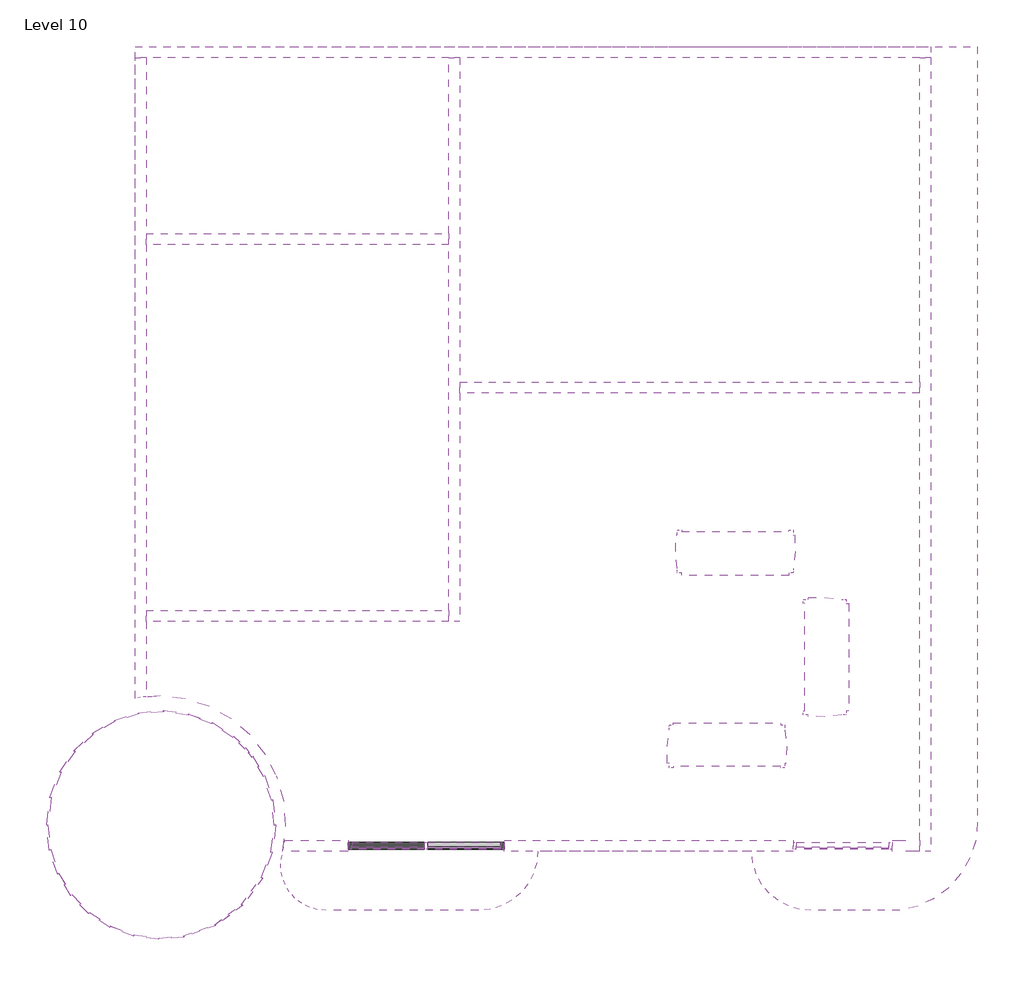
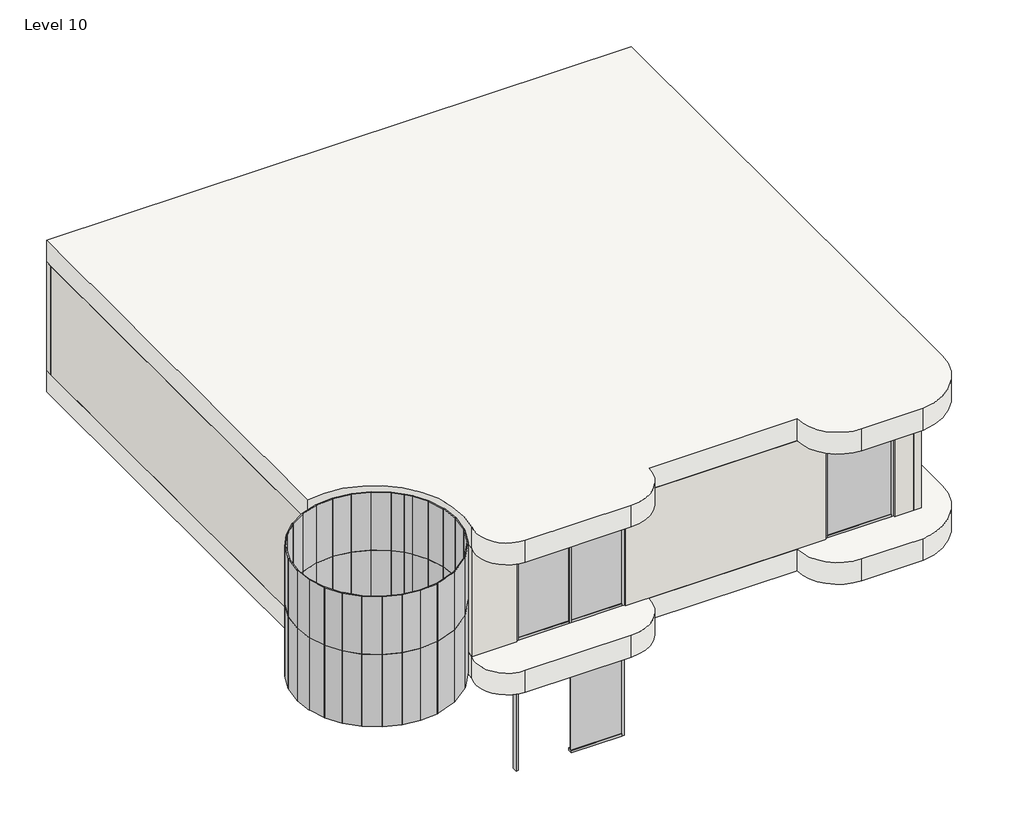
# One storey, incomplete: 60 plates, 15 members, 10 walls, 3 furniture elements, 2 slabs.
"""IFC4 building model written with IfcOpenShell, lengths in millimetres."""

from ifc_helpers import new_model, si_unit, point, frame, frame_2d, origin, place, context, project, spatial, polyline, circle_curve, trimmed, segment, composite_curve, outline, extrude, faceted_brep, transform, mapped, element, save
from ifc_brep_helpers import plane_surface, revolved_surface, advanced_brep
from components import furniture_aff9b2fb, member_eaba9652, member_3f395ae9, member_0c868e12, member_7bc42366, system_panel_glazed_f1c144f9, system_panel_glazed_8ed2b2ee, system_panel_glazed_c7815b78, system_panel_glazed_220ba5f3, system_panel_glazed_11fb153e, system_panel_glazed_2f540b85, system_panel_glazed_4848e608, system_panel_glazed_8b35a0ff, system_panel_glazed_87282c25, system_panel_glazed_6d1bb68c, system_panel_glazed_cb3ffd69, system_panel_glazed_404d015f, system_panel_glazed_7b556abe, system_panel_glazed_370bf902

model = new_model("IFC4")

# Units and contexts
model_context = context("Model", 3, world=origin())
ifc_project = project(units=[si_unit("LENGTHUNIT", "METRE", prefix="MILLI")], contexts=[model_context])

# Site, building, storey
site = spatial("IfcSite", under=ifc_project)
building = spatial("IfcBuilding", under=site)
storey = spatial("IfcBuildingStorey", under=building, Name="Level 10", Elevation=27432.0)

# Furniture
placement = place(None, origin())
furniture_shape = furniture_aff9b2fb(model_context)
element("IfcFurniture", 1, ObjectType="Sofa-Pensi : 84\"", at=placement, inside=storey, context=model_context, shape_type="MappedRepresentation", body=[
    mapped(furniture_shape, transform((-2244.8524991, 3650.1964615, 29260.8), x_axis=(1.0, 0.0, 0.0), y_axis=(0.0, 1.0, 0.0), z_axis=(0.0, 0.0, 1.0))),
])
element("IfcFurniture", 2, ObjectType="Sofa-Pensi : 84\"", at=placement, inside=storey, context=model_context, shape_type="MappedRepresentation", body=[
    mapped(furniture_shape, transform((-12.736413, 1720.492712, 29260.8), x_axis=(0.0, 1.0, 0.0), y_axis=(-1.0, 0.0, 0.0), z_axis=(0.0, 0.0, 1.0))),
])
element("IfcFurniture", 3, ObjectType="Sofa-Pensi : 84\"", at=placement, inside=storey, context=model_context, shape_type="MappedRepresentation", body=[
    mapped(furniture_shape, transform((-1840.0399991, 648.4161336, 29260.8), x_axis=(-1.0, 0.0, 0.0), y_axis=(0.0, -1.0, 0.0), z_axis=(0.0, 0.0, 1.0))),
])

# Members
member_shape = member_eaba9652(model_context)
element("IfcMember", 4, ObjectType="Rectangular Mullion : 2.5\" x 5\" rectangular", at=placement, inside=storey, context=model_context, shape_type="MappedRepresentation", body=[
    mapped(member_shape, transform((-7672.5789001, -1482.8937024, 29260.8), x_axis=(-1.0, 0.0, 0.0), y_axis=(0.0, 1.0, 0.0), z_axis=(0.0, 0.0, -1.0))),
])
member_2_shape = member_3f395ae9(model_context)
element("IfcMember", 5, ObjectType="Rectangular Mullion : 2.5\" x 5\" rectangular", at=placement, inside=storey, context=model_context, shape_type="MappedRepresentation", body=[
    mapped(member_2_shape, transform((-9111.7115512, -1482.8937024, 25603.2), x_axis=(-1.0, 0.0, 0.0), y_axis=(0.0, 1.0, 0.0), z_axis=(0.0, 0.0, -1.0))),
])
element("IfcMember", 6, ObjectType="Rectangular Mullion : 2.5\" x 5\" rectangular", at=placement, inside=storey, context=model_context, shape_type="MappedRepresentation", body=[
    mapped(member_2_shape, transform((-9111.7115512, -1482.8937024, 29260.8), x_axis=(-1.0, 0.0, 0.0), y_axis=(0.0, 1.0, 0.0), z_axis=(0.0, 0.0, -1.0))),
])
element("IfcMember", 7, ObjectType="Rectangular Mullion : 2.5\" x 5\" rectangular", at=placement, inside=storey, context=model_context, shape_type="MappedRepresentation", body=[
    mapped(member_2_shape, transform((-899.4462491, -1482.8937024, 29260.8), x_axis=(-1.0, 0.0, 0.0), y_axis=(0.0, 1.0, 0.0), z_axis=(0.0, 0.0, -1.0))),
])
element("IfcMember", 8, ObjectType="Rectangular Mullion : 2.5\" x 5\" rectangular", at=placement, inside=storey, context=model_context, shape_type="MappedRepresentation", body=[
    mapped(member_2_shape, transform((-6233.4462491, -1482.8937024, 28651.2), x_axis=(1.0, 0.0, 0.0), y_axis=(0.0, 1.0, 0.0), z_axis=(0.0, 0.0, 1.0))),
])
element("IfcMember", 9, ObjectType="Rectangular Mullion : 2.5\" x 5\" rectangular", at=placement, inside=storey, context=model_context, shape_type="MappedRepresentation", body=[
    mapped(member_2_shape, transform((-6233.4462491, -1482.8937024, 32308.8), x_axis=(1.0, 0.0, 0.0), y_axis=(0.0, 1.0, 0.0), z_axis=(0.0, 0.0, 1.0))),
])
element("IfcMember", 10, ObjectType="Rectangular Mullion : 2.5\" x 5\" rectangular", at=placement, inside=storey, context=model_context, shape_type="MappedRepresentation", body=[
    mapped(member_2_shape, transform((929.3537509, -1482.8937024, 32308.8), x_axis=(1.0, 0.0, 0.0), y_axis=(0.0, 1.0, 0.0), z_axis=(0.0, 0.0, 1.0))),
])
member_3_shape = member_0c868e12(model_context)
element("IfcMember", 11, ObjectType="Rectangular Mullion : 2.5\" x 5\" rectangular", at=placement, inside=storey, context=model_context, shape_type="MappedRepresentation", body=[
    mapped(member_3_shape, transform((-9048.2115512, -1482.8937024, 28651.2), x_axis=(0.0, 0.0, 1.0), y_axis=(0.0, 1.0, 0.0), z_axis=(-1.0, 0.0, 0.0))),
])
element("IfcMember", 12, ObjectType="Rectangular Mullion : 2.5\" x 5\" rectangular", at=placement, inside=storey, context=model_context, shape_type="MappedRepresentation", body=[
    mapped(member_3_shape, transform((-9048.2115512, -1482.8937024, 32308.8), x_axis=(0.0, 0.0, 1.0), y_axis=(0.0, 1.0, 0.0), z_axis=(-1.0, 0.0, 0.0))),
])
element("IfcMember", 13, ObjectType="Rectangular Mullion : 2.5\" x 5\" rectangular", at=placement, inside=storey, context=model_context, shape_type="MappedRepresentation", body=[
    mapped(member_3_shape, transform((-7640.8289001, -1482.8937024, 32308.8), x_axis=(0.0, 0.0, 1.0), y_axis=(0.0, 1.0, 0.0), z_axis=(-1.0, 0.0, 0.0))),
])
element("IfcMember", 14, ObjectType="Rectangular Mullion : 2.5\" x 5\" rectangular", at=placement, inside=storey, context=model_context, shape_type="MappedRepresentation", body=[
    mapped(member_3_shape, transform((-6296.9462491, -1482.8937024, 25603.2), x_axis=(0.0, 0.0, -1.0), y_axis=(0.0, 1.0, 0.0), z_axis=(1.0, 0.0, 0.0))),
])
element("IfcMember", 15, ObjectType="Rectangular Mullion : 2.5\" x 5\" rectangular", at=placement, inside=storey, context=model_context, shape_type="MappedRepresentation", body=[
    mapped(member_3_shape, transform((-6296.9462491, -1482.8937024, 29260.8), x_axis=(0.0, 0.0, -1.0), y_axis=(0.0, 1.0, 0.0), z_axis=(1.0, 0.0, 0.0))),
])
element("IfcMember", 16, ObjectType="Rectangular Mullion : 2.5\" x 5\" rectangular", at=placement, inside=storey, context=model_context, shape_type="MappedRepresentation", body=[
    mapped(member_3_shape, transform((-7704.3289001, -1482.8937024, 29260.8), x_axis=(0.0, 0.0, -1.0), y_axis=(0.0, 1.0, 0.0), z_axis=(1.0, 0.0, 0.0))),
])
member_4_shape = member_7bc42366(model_context)
element("IfcMember", 17, ObjectType="Rectangular Mullion : 2.5\" x 5\" rectangular", at=placement, inside=storey, context=model_context, shape_type="MappedRepresentation", body=[
    mapped(member_4_shape, transform((-835.9462491, -1482.8937024, 32308.8), x_axis=(0.0, 0.0, 1.0), y_axis=(0.0, 1.0, 0.0), z_axis=(-1.0, 0.0, 0.0))),
])
element("IfcMember", 18, ObjectType="Rectangular Mullion : 2.5\" x 5\" rectangular", at=placement, inside=storey, context=model_context, shape_type="MappedRepresentation", body=[
    mapped(member_4_shape, transform((865.8537509, -1482.8937024, 29260.8), x_axis=(0.0, 0.0, -1.0), y_axis=(0.0, 1.0, 0.0), z_axis=(1.0, 0.0, 0.0))),
])

# Plates
system_panel_glazed_shape = system_panel_glazed_f1c144f9(model_context)
element("IfcPlate", 19, ObjectType="System Panel : Glazed", at=placement, inside=storey, context=model_context, shape_type="MappedRepresentation", body=[
    mapped(system_panel_glazed_shape, transform((-14541.9245022, -346.5978939, 29260.8), x_axis=(-0.3551689475306269, -0.9348021281051873, 0.0), y_axis=(0.9348021281051873, -0.3551689475306269, 0.0), z_axis=(0.0, 0.0, 1.0))),
])
element("IfcPlate", 20, ObjectType="System Panel : Glazed", at=placement, inside=storey, context=model_context, shape_type="MappedRepresentation", body=[
    mapped(system_panel_glazed_shape, transform((-10582.1178502, -1851.0877948, 29260.8), x_axis=(0.35516894753064066, 0.934802128105182, 0.0), y_axis=(-0.934802128105182, 0.35516894753064066, 0.0), z_axis=(0.0, 0.0, 1.0))),
])
element("IfcPlate", 21, ObjectType="System Panel : Glazed", at=placement, inside=storey, context=model_context, shape_type="MappedRepresentation", body=[
    mapped(system_panel_glazed_shape, transform((-10459.5232171, -1354.5613954, 29260.8), x_axis=(0.12073632210407237, 0.9926846128175765, 0.0), y_axis=(-0.9926846128175765, 0.12073632210407237, 0.0), z_axis=(0.0, 0.0, 1.0))),
])
element("IfcPlate", 22, ObjectType="System Panel : Glazed", at=placement, inside=storey, context=model_context, shape_type="MappedRepresentation", body=[
    mapped(system_panel_glazed_shape, transform((-14664.5191354, -843.1242933, 29260.8), x_axis=(-0.12073632210406239, -0.9926846128175777, 0.0), y_axis=(0.9926846128175777, -0.12073632210406239, 0.0), z_axis=(0.0, 0.0, 1.0))),
])
system_panel_glazed_2_shape = system_panel_glazed_8ed2b2ee(model_context)
element("IfcPlate", 23, ObjectType="System Panel : Glazed", at=placement, inside=storey, context=model_context, shape_type="MappedRepresentation", body=[
    mapped(system_panel_glazed_2_shape, transform((-11841.3777431, -3082.3793017, 29260.8), x_axis=(0.9398911711666007, 0.3414741371803665, 0.0), y_axis=(-0.3414741371803665, 0.9398911711666007, 0.0), z_axis=(0.0, 0.0, 1.0))),
])
element("IfcPlate", 24, ObjectType="System Panel : Glazed", at=placement, inside=storey, context=model_context, shape_type="MappedRepresentation", body=[
    mapped(system_panel_glazed_2_shape, transform((-10858.9635423, -2345.1728692, 29260.8), x_axis=(0.5905687200141164, 0.8069873524045393, 0.0), y_axis=(-0.8069873524045393, 0.5905687200141164, 0.0), z_axis=(0.0, 0.0, 1.0))),
])
element("IfcPlate", 25, ObjectType="System Panel : Glazed", at=placement, inside=storey, context=model_context, shape_type="MappedRepresentation", body=[
    mapped(system_panel_glazed_2_shape, transform((-11295.3522982, -2786.8279712, 29260.8), x_axis=(0.7998453025525061, 0.6002062078858317, 0.0), y_axis=(-0.6002062078858317, 0.7998453025525061, 0.0), z_axis=(0.0, 0.0, 1.0))),
])
system_panel_glazed_3_shape = system_panel_glazed_c7815b78(model_context)
element("IfcPlate", 26, ObjectType="System Panel : Glazed", at=placement, inside=storey, context=model_context, shape_type="MappedRepresentation", body=[
    mapped(system_panel_glazed_3_shape, transform((-10454.4737362, -864.5204039, 29260.8), x_axis=(-0.11050163420416614, 0.993875942378227, 0.0), y_axis=(-0.993875942378227, -0.11050163420416614, 0.0), z_axis=(0.0, 0.0, 1.0))),
])
element("IfcPlate", 27, ObjectType="System Panel : Glazed", at=placement, inside=storey, context=model_context, shape_type="MappedRepresentation", body=[
    mapped(system_panel_glazed_3_shape, transform((-14669.5686163, -1333.1652848, 29260.8), x_axis=(0.11050163420415136, -0.9938759423782286, 0.0), y_axis=(0.9938759423782286, 0.11050163420415136, 0.0), z_axis=(0.0, 0.0, 1.0))),
])
element("IfcPlate", 28, ObjectType="System Panel : Glazed", at=placement, inside=storey, context=model_context, shape_type="MappedRepresentation", body=[
    mapped(system_panel_glazed_3_shape, transform((-11410.1424167, 681.5611944, 29260.8), x_axis=(-0.8396018558176894, 0.5432022861766066, 0.0), y_axis=(-0.5432022861766066, -0.8396018558176894, 0.0), z_axis=(0.0, 0.0, 1.0))),
])
element("IfcPlate", 29, ObjectType="System Panel : Glazed", at=placement, inside=storey, context=model_context, shape_type="MappedRepresentation", body=[
    mapped(system_panel_glazed_3_shape, transform((-13212.0893695, 919.590846, 29260.8), x_axis=(-0.9518517343814786, -0.3065587639506839, 0.0), y_axis=(0.3065587639506839, -0.9518517343814786, 0.0), z_axis=(0.0, 0.0, 1.0))),
])
element("IfcPlate", 30, ObjectType="System Panel : Glazed", at=placement, inside=storey, context=model_context, shape_type="MappedRepresentation", body=[
    mapped(system_panel_glazed_3_shape, transform((-12839.7224363, -3201.1142893, 29260.8), x_axis=(0.9913878918151698, -0.1309581916577702, 0.0), y_axis=(0.1309581916577702, 0.9913878918151698, 0.0), z_axis=(0.0, 0.0, 1.0))),
])
element("IfcPlate", 31, ObjectType="System Panel : Glazed", at=placement, inside=storey, context=model_context, shape_type="MappedRepresentation", body=[
    mapped(system_panel_glazed_3_shape, transform((-14365.783041, -2213.7896382, 29260.8), x_axis=(0.5257859322352114, -0.8506169252157811, 0.0), y_axis=(0.8506169252157811, 0.5257859322352114, 0.0), z_axis=(0.0, 0.0, 1.0))),
])
element("IfcPlate", 32, ObjectType="System Panel : Glazed", at=placement, inside=storey, context=model_context, shape_type="MappedRepresentation", body=[
    mapped(system_panel_glazed_3_shape, transform((-13713.8999358, -2879.2468831, 29260.8), x_axis=(0.8396018558176805, -0.5432022861766201, 0.0), y_axis=(0.5432022861766201, 0.8396018558176805, 0.0), z_axis=(0.0, 0.0, 1.0))),
])
element("IfcPlate", 33, ObjectType="System Panel : Glazed", at=placement, inside=storey, context=model_context, shape_type="MappedRepresentation", body=[
    mapped(system_panel_glazed_3_shape, transform((-14014.4059364, 446.2272921, 29260.8), x_axis=(-0.7286232370002992, -0.6849147235263715, 0.0), y_axis=(0.6849147235263715, -0.7286232370002992, 0.0), z_axis=(0.0, 0.0, 1.0))),
])
element("IfcPlate", 34, ObjectType="System Panel : Glazed", at=placement, inside=storey, context=model_context, shape_type="MappedRepresentation", body=[
    mapped(system_panel_glazed_3_shape, transform((-12284.3199161, 1003.4286006, 29260.8), x_axis=(-0.9913878918151723, 0.13095819165775144, 0.0), y_axis=(-0.13095819165775144, -0.9913878918151723, 0.0), z_axis=(0.0, 0.0, 1.0))),
])
element("IfcPlate", 35, ObjectType="System Panel : Glazed", at=placement, inside=storey, context=model_context, shape_type="MappedRepresentation", body=[
    mapped(system_panel_glazed_3_shape, transform((-12752.8652893, 1013.0855973, 29260.8), x_axis=(-0.9959419324521102, -0.08999815100076568, 0.0), y_axis=(0.08999815100076568, -0.9959419324521102, 0.0), z_axis=(0.0, 0.0, 1.0))),
])
element("IfcPlate", 36, ObjectType="System Panel : Glazed", at=placement, inside=storey, context=model_context, shape_type="MappedRepresentation", body=[
    mapped(system_panel_glazed_3_shape, transform((-11829.3381514, 891.0915272, 29260.8), x_axis=(-0.9384120429483949, 0.3455182160891376, 0.0), y_axis=(-0.3455182160891376, -0.9384120429483949, 0.0), z_axis=(0.0, 0.0, 1.0))),
])
element("IfcPlate", 37, ObjectType="System Panel : Glazed", at=placement, inside=storey, context=model_context, shape_type="MappedRepresentation", body=[
    mapped(system_panel_glazed_3_shape, transform((-10557.4115054, -407.3204039, 29260.8), x_axis=(-0.3261077326604367, 0.9453326116764772, 0.0), y_axis=(-0.9453326116764772, -0.3261077326604367, 0.0), z_axis=(0.0, 0.0, 1.0))),
])
element("IfcPlate", 38, ObjectType="System Panel : Glazed", at=placement, inside=storey, context=model_context, shape_type="MappedRepresentation", body=[
    mapped(system_panel_glazed_3_shape, transform((-12371.1770631, -3210.771286, 29260.8), x_axis=(0.9959419324521115, 0.08999815100075001, 0.0), y_axis=(-0.08999815100075001, 0.9959419324521115, 0.0), z_axis=(0.0, 0.0, 1.0))),
])
element("IfcPlate", 39, ObjectType="System Panel : Glazed", at=placement, inside=storey, context=model_context, shape_type="MappedRepresentation", body=[
    mapped(system_panel_glazed_3_shape, transform((-13294.7042011, -3088.7772159, 29260.8), x_axis=(0.9384120429483891, -0.34551821608915334, 0.0), y_axis=(0.34551821608915334, 0.9384120429483891, 0.0), z_axis=(0.0, 0.0, 1.0))),
])
element("IfcPlate", 40, ObjectType="System Panel : Glazed", at=placement, inside=storey, context=model_context, shape_type="MappedRepresentation", body=[
    mapped(system_panel_glazed_3_shape, transform((-14076.8350959, -2582.7572647, 29260.8), x_axis=(0.6997834615185511, -0.7143550286692988, 0.0), y_axis=(0.7143550286692988, 0.6997834615185511, 0.0), z_axis=(0.0, 0.0, 1.0))),
])
element("IfcPlate", 41, ObjectType="System Panel : Glazed", at=placement, inside=storey, context=model_context, shape_type="MappedRepresentation", body=[
    mapped(system_panel_glazed_3_shape, transform((-14566.6308471, -1790.3652848, 29260.8), x_axis=(0.32610773266042153, -0.9453326116764824, 0.0), y_axis=(0.9453326116764824, 0.32610773266042153, 0.0), z_axis=(0.0, 0.0, 1.0))),
])
element("IfcPlate", 42, ObjectType="System Panel : Glazed", at=placement, inside=storey, context=model_context, shape_type="MappedRepresentation", body=[
    mapped(system_panel_glazed_3_shape, transform((-14318.3113206, 89.4787227, 29260.8), x_axis=(-0.5603879632167612, -0.8282302401396425, 0.0), y_axis=(0.8282302401396425, -0.5603879632167612, 0.0), z_axis=(0.0, 0.0, 1.0))),
])
element("IfcPlate", 43, ObjectType="System Panel : Glazed", at=placement, inside=storey, context=model_context, shape_type="MappedRepresentation", body=[
    mapped(system_panel_glazed_3_shape, transform((-13639.5625299, 727.5108588, 29260.8), x_axis=(-0.8612707706620224, -0.5081462974412448, 0.0), y_axis=(0.5081462974412448, -0.8612707706620224, 0.0), z_axis=(0.0, 0.0, 1.0))),
])
system_panel_glazed_4_shape = system_panel_glazed_220ba5f3(model_context)
element("IfcPlate", 44, ObjectType="System Panel : Glazed", at=placement, inside=storey, context=model_context, shape_type="MappedRepresentation", body=[
    mapped(system_panel_glazed_4_shape, transform((-10742.3305673, -4.7597883, 29260.8), x_axis=(-0.5152811917631037, 0.8570211744263939, 0.0), y_axis=(-0.8570211744263939, -0.5152811917631037, 0.0), z_axis=(0.0, 0.0, 1.0))),
])
system_panel_glazed_5_shape = system_panel_glazed_11fb153e(model_context)
element("IfcPlate", 45, ObjectType="System Panel : Glazed", at=placement, inside=storey, context=model_context, shape_type="MappedRepresentation", body=[
    mapped(system_panel_glazed_5_shape, transform((-11098.0043985, 445.2241463, 29260.8), x_axis=(-0.7256671855033587, 0.6880458821064435, 0.0), y_axis=(-0.6880458821064435, -0.7256671855033587, 0.0), z_axis=(0.0, 0.0, 1.0))),
])
system_panel_glazed_6_shape = system_panel_glazed_2f540b85(model_context)
element("IfcPlate", 46, ObjectType="System Panel : Glazed", at=placement, inside=storey, context=model_context, shape_type="MappedRepresentation", body=[
    mapped(system_panel_glazed_6_shape, transform((-10917.0903061, 255.9395759, 29260.8), x_axis=(-0.6357445726375757, 0.7718995001694627, 0.0), y_axis=(-0.7718995001694627, -0.6357445726375757, 0.0), z_axis=(0.0, 0.0, 1.0))),
])
system_panel_glazed_7_shape = system_panel_glazed_4848e608(model_context)
element("IfcPlate", 47, ObjectType="System Panel : Glazed", at=placement, inside=storey, context=model_context, shape_type="MappedRepresentation", body=[
    mapped(system_panel_glazed_7_shape, transform((-14669.5686163, -1333.1652848, 31292.8), x_axis=(0.11050163420415136, -0.9938759423782286, 0.0), y_axis=(0.9938759423782286, 0.11050163420415136, 0.0), z_axis=(0.0, 0.0, 1.0))),
])
element("IfcPlate", 48, ObjectType="System Panel : Glazed", at=placement, inside=storey, context=model_context, shape_type="MappedRepresentation", body=[
    mapped(system_panel_glazed_7_shape, transform((-14365.783041, -2213.7896382, 31292.8), x_axis=(0.5257859322352114, -0.8506169252157811, 0.0), y_axis=(0.8506169252157811, 0.5257859322352114, 0.0), z_axis=(0.0, 0.0, 1.0))),
])
element("IfcPlate", 49, ObjectType="System Panel : Glazed", at=placement, inside=storey, context=model_context, shape_type="MappedRepresentation", body=[
    mapped(system_panel_glazed_7_shape, transform((-13713.8999358, -2879.2468831, 31292.8), x_axis=(0.8396018558176805, -0.5432022861766201, 0.0), y_axis=(0.5432022861766201, 0.8396018558176805, 0.0), z_axis=(0.0, 0.0, 1.0))),
])
element("IfcPlate", 50, ObjectType="System Panel : Glazed", at=placement, inside=storey, context=model_context, shape_type="MappedRepresentation", body=[
    mapped(system_panel_glazed_7_shape, transform((-12839.7224363, -3201.1142893, 31292.8), x_axis=(0.9913878918151698, -0.13095819165777017, 0.0), y_axis=(0.13095819165777017, 0.9913878918151698, 0.0), z_axis=(0.0, 0.0, 1.0))),
])
element("IfcPlate", 51, ObjectType="System Panel : Glazed", at=placement, inside=storey, context=model_context, shape_type="MappedRepresentation", body=[
    mapped(system_panel_glazed_7_shape, transform((-12371.1770631, -3210.771286, 31292.8), x_axis=(0.9959419324521115, 0.08999815100075001, 0.0), y_axis=(-0.08999815100075001, 0.9959419324521115, 0.0), z_axis=(0.0, 0.0, 1.0))),
])
element("IfcPlate", 52, ObjectType="System Panel : Glazed", at=placement, inside=storey, context=model_context, shape_type="MappedRepresentation", body=[
    mapped(system_panel_glazed_7_shape, transform((-13294.7042011, -3088.7772159, 31292.8), x_axis=(0.9384120429483891, -0.34551821608915334, 0.0), y_axis=(0.34551821608915334, 0.9384120429483891, 0.0), z_axis=(0.0, 0.0, 1.0))),
])
element("IfcPlate", 53, ObjectType="System Panel : Glazed", at=placement, inside=storey, context=model_context, shape_type="MappedRepresentation", body=[
    mapped(system_panel_glazed_7_shape, transform((-14076.8350959, -2582.7572647, 31292.8), x_axis=(0.6997834615185511, -0.7143550286692988, 0.0), y_axis=(0.7143550286692988, 0.6997834615185511, 0.0), z_axis=(0.0, 0.0, 1.0))),
])
element("IfcPlate", 54, ObjectType="System Panel : Glazed", at=placement, inside=storey, context=model_context, shape_type="MappedRepresentation", body=[
    mapped(system_panel_glazed_7_shape, transform((-14566.6308471, -1790.3652848, 31292.8), x_axis=(0.32610773266042153, -0.9453326116764824, 0.0), y_axis=(0.9453326116764824, 0.32610773266042153, 0.0), z_axis=(0.0, 0.0, 1.0))),
])
element("IfcPlate", 55, ObjectType="System Panel : Glazed", at=placement, inside=storey, context=model_context, shape_type="MappedRepresentation", body=[
    mapped(system_panel_glazed_7_shape, transform((-10454.4737362, -864.5204039, 31292.8), x_axis=(-0.11050163420416614, 0.993875942378227, 0.0), y_axis=(-0.993875942378227, -0.11050163420416614, 0.0), z_axis=(0.0, 0.0, 1.0))),
])
element("IfcPlate", 56, ObjectType="System Panel : Glazed", at=placement, inside=storey, context=model_context, shape_type="MappedRepresentation", body=[
    mapped(system_panel_glazed_7_shape, transform((-10557.4115054, -407.3204039, 31292.8), x_axis=(-0.3261077326604368, 0.9453326116764772, 0.0), y_axis=(-0.9453326116764772, -0.3261077326604368, 0.0), z_axis=(0.0, 0.0, 1.0))),
])
element("IfcPlate", 57, ObjectType="System Panel : Glazed", at=placement, inside=storey, context=model_context, shape_type="MappedRepresentation", body=[
    mapped(system_panel_glazed_7_shape, transform((-11410.1424167, 681.5611944, 31292.8), x_axis=(-0.8396018558176894, 0.5432022861766066, 0.0), y_axis=(-0.5432022861766066, -0.8396018558176894, 0.0), z_axis=(0.0, 0.0, 1.0))),
])
element("IfcPlate", 58, ObjectType="System Panel : Glazed", at=placement, inside=storey, context=model_context, shape_type="MappedRepresentation", body=[
    mapped(system_panel_glazed_7_shape, transform((-11829.3381514, 891.0915272, 31292.8), x_axis=(-0.9384120429483949, 0.3455182160891376, 0.0), y_axis=(-0.3455182160891376, -0.9384120429483949, 0.0), z_axis=(0.0, 0.0, 1.0))),
])
element("IfcPlate", 59, ObjectType="System Panel : Glazed", at=placement, inside=storey, context=model_context, shape_type="MappedRepresentation", body=[
    mapped(system_panel_glazed_7_shape, transform((-12284.3199161, 1003.4286006, 31292.8), x_axis=(-0.9913878918151723, 0.1309581916577514, 0.0), y_axis=(-0.1309581916577514, -0.9913878918151723, 0.0), z_axis=(0.0, 0.0, 1.0))),
])
element("IfcPlate", 60, ObjectType="System Panel : Glazed", at=placement, inside=storey, context=model_context, shape_type="MappedRepresentation", body=[
    mapped(system_panel_glazed_7_shape, transform((-12752.8652893, 1013.0855973, 31292.8), x_axis=(-0.9959419324521102, -0.08999815100076568, 0.0), y_axis=(0.08999815100076568, -0.9959419324521102, 0.0), z_axis=(0.0, 0.0, 1.0))),
])
element("IfcPlate", 61, ObjectType="System Panel : Glazed", at=placement, inside=storey, context=model_context, shape_type="MappedRepresentation", body=[
    mapped(system_panel_glazed_7_shape, transform((-13212.0893695, 919.590846, 31292.8), x_axis=(-0.9518517343814786, -0.3065587639506839, 0.0), y_axis=(0.3065587639506839, -0.9518517343814786, 0.0), z_axis=(0.0, 0.0, 1.0))),
])
element("IfcPlate", 62, ObjectType="System Panel : Glazed", at=placement, inside=storey, context=model_context, shape_type="MappedRepresentation", body=[
    mapped(system_panel_glazed_7_shape, transform((-13639.5625299, 727.5108588, 31292.8), x_axis=(-0.8612707706620223, -0.508146297441245, 0.0), y_axis=(0.508146297441245, -0.8612707706620223, 0.0), z_axis=(0.0, 0.0, 1.0))),
])
element("IfcPlate", 63, ObjectType="System Panel : Glazed", at=placement, inside=storey, context=model_context, shape_type="MappedRepresentation", body=[
    mapped(system_panel_glazed_7_shape, transform((-14014.4059364, 446.2272921, 31292.8), x_axis=(-0.7286232370002992, -0.6849147235263715, 0.0), y_axis=(0.6849147235263715, -0.7286232370002992, 0.0), z_axis=(0.0, 0.0, 1.0))),
])
element("IfcPlate", 64, ObjectType="System Panel : Glazed", at=placement, inside=storey, context=model_context, shape_type="MappedRepresentation", body=[
    mapped(system_panel_glazed_7_shape, transform((-14318.3113206, 89.4787227, 31292.8), x_axis=(-0.5603879632167612, -0.8282302401396425, 0.0), y_axis=(0.8282302401396425, -0.5603879632167612, 0.0), z_axis=(0.0, 0.0, 1.0))),
])
system_panel_glazed_8_shape = system_panel_glazed_8b35a0ff(model_context)
element("IfcPlate", 65, ObjectType="System Panel : Glazed", at=placement, inside=storey, context=model_context, shape_type="MappedRepresentation", body=[
    mapped(system_panel_glazed_8_shape, transform((-10742.3305673, -4.7597883, 31292.8), x_axis=(-0.5152811917631037, 0.8570211744263939, 0.0), y_axis=(-0.8570211744263939, -0.5152811917631037, 0.0), z_axis=(0.0, 0.0, 1.0))),
])
system_panel_glazed_9_shape = system_panel_glazed_87282c25(model_context)
element("IfcPlate", 66, ObjectType="System Panel : Glazed", at=placement, inside=storey, context=model_context, shape_type="MappedRepresentation", body=[
    mapped(system_panel_glazed_9_shape, transform((-10917.0903061, 255.9395759, 31292.8), x_axis=(-0.6357445726375757, 0.7718995001694627, 0.0), y_axis=(-0.7718995001694627, -0.6357445726375757, 0.0), z_axis=(0.0, 0.0, 1.0))),
])
system_panel_glazed_10_shape = system_panel_glazed_6d1bb68c(model_context)
element("IfcPlate", 67, ObjectType="System Panel : Glazed", at=placement, inside=storey, context=model_context, shape_type="MappedRepresentation", body=[
    mapped(system_panel_glazed_10_shape, transform((-11098.0043985, 445.2241463, 31292.8), x_axis=(-0.7256671855033587, 0.6880458821064435, 0.0), y_axis=(-0.6880458821064435, -0.7256671855033587, 0.0), z_axis=(0.0, 0.0, 1.0))),
])
system_panel_glazed_11_shape = system_panel_glazed_cb3ffd69(model_context)
element("IfcPlate", 68, ObjectType="System Panel : Glazed", at=placement, inside=storey, context=model_context, shape_type="MappedRepresentation", body=[
    mapped(system_panel_glazed_11_shape, transform((-10582.1178502, -1851.0877948, 31292.8), x_axis=(0.35516894753064066, 0.934802128105182, 0.0), y_axis=(-0.934802128105182, 0.35516894753064066, 0.0), z_axis=(0.0, 0.0, 1.0))),
])
element("IfcPlate", 69, ObjectType="System Panel : Glazed", at=placement, inside=storey, context=model_context, shape_type="MappedRepresentation", body=[
    mapped(system_panel_glazed_11_shape, transform((-10459.5232171, -1354.5613954, 31292.8), x_axis=(0.1207363221040724, 0.9926846128175765, 0.0), y_axis=(-0.9926846128175765, 0.1207363221040724, 0.0), z_axis=(0.0, 0.0, 1.0))),
])
element("IfcPlate", 70, ObjectType="System Panel : Glazed", at=placement, inside=storey, context=model_context, shape_type="MappedRepresentation", body=[
    mapped(system_panel_glazed_11_shape, transform((-14541.9245022, -346.5978939, 31292.8), x_axis=(-0.3551689475306269, -0.9348021281051873, 0.0), y_axis=(0.9348021281051873, -0.3551689475306269, 0.0), z_axis=(0.0, 0.0, 1.0))),
])
element("IfcPlate", 71, ObjectType="System Panel : Glazed", at=placement, inside=storey, context=model_context, shape_type="MappedRepresentation", body=[
    mapped(system_panel_glazed_11_shape, transform((-14664.5191354, -843.1242933, 31292.8), x_axis=(-0.1207363221040624, -0.9926846128175777, 0.0), y_axis=(0.9926846128175777, -0.1207363221040624, 0.0), z_axis=(0.0, 0.0, 1.0))),
])
system_panel_glazed_12_shape = system_panel_glazed_404d015f(model_context)
element("IfcPlate", 72, ObjectType="System Panel : Glazed", at=placement, inside=storey, context=model_context, shape_type="MappedRepresentation", body=[
    mapped(system_panel_glazed_12_shape, transform((-11841.3777431, -3082.3793017, 31292.8), x_axis=(0.9398911711666007, 0.3414741371803665, 0.0), y_axis=(-0.3414741371803665, 0.9398911711666007, 0.0), z_axis=(0.0, 0.0, 1.0))),
])
element("IfcPlate", 73, ObjectType="System Panel : Glazed", at=placement, inside=storey, context=model_context, shape_type="MappedRepresentation", body=[
    mapped(system_panel_glazed_12_shape, transform((-10858.9635423, -2345.1728692, 31292.8), x_axis=(0.5905687200141164, 0.8069873524045393, 0.0), y_axis=(-0.8069873524045393, 0.5905687200141164, 0.0), z_axis=(0.0, 0.0, 1.0))),
])
element("IfcPlate", 74, ObjectType="System Panel : Glazed", at=placement, inside=storey, context=model_context, shape_type="MappedRepresentation", body=[
    mapped(system_panel_glazed_12_shape, transform((-11295.3522982, -2786.8279712, 31292.8), x_axis=(0.7998453025525062, 0.6002062078858316, 0.0), y_axis=(-0.6002062078858316, 0.7998453025525062, 0.0), z_axis=(0.0, 0.0, 1.0))),
])
system_panel_glazed_13_shape = system_panel_glazed_7b556abe(model_context)
element("IfcPlate", 75, ObjectType="System Panel : Glazed", at=placement, inside=storey, context=model_context, shape_type="MappedRepresentation", body=[
    mapped(system_panel_glazed_13_shape, transform((-6968.8875746, -1482.8937024, 25666.7), x_axis=(-1.0, 0.0, 0.0), y_axis=(0.0, -1.0, 0.0), z_axis=(0.0, 0.0, 1.0))),
])
element("IfcPlate", 76, ObjectType="System Panel : Glazed", at=placement, inside=storey, context=model_context, shape_type="MappedRepresentation", body=[
    mapped(system_panel_glazed_13_shape, transform((-6968.8875746, -1482.8937024, 29324.3), x_axis=(-1.0, 0.0, 0.0), y_axis=(0.0, -1.0, 0.0), z_axis=(0.0, 0.0, 1.0))),
])
element("IfcPlate", 77, ObjectType="System Panel : Glazed", at=placement, inside=storey, context=model_context, shape_type="MappedRepresentation", body=[
    mapped(system_panel_glazed_13_shape, transform((-8376.2702257, -1482.8937024, 29324.3), x_axis=(-1.0, 0.0, 0.0), y_axis=(0.0, -1.0, 0.0), z_axis=(0.0, 0.0, 1.0))),
])
system_panel_glazed_14_shape = system_panel_glazed_370bf902(model_context)
element("IfcPlate", 78, ObjectType="System Panel : Glazed", at=placement, inside=storey, context=model_context, shape_type="MappedRepresentation", body=[
    mapped(system_panel_glazed_14_shape, transform((14.9537509, -1482.8937024, 29324.3), x_axis=(-1.0, 0.0, 0.0), y_axis=(0.0, -1.0, 0.0), z_axis=(0.0, 0.0, 1.0))),
])

# Slabs
element("IfcSlab", 79, ObjectType="Generic - 2'", at=placement, inside=storey, context=model_context, shape_type="SweptSolid", body=[
    extrude(outline(composite_curve([segment(polyline([(2504.1537509, 13274.5062976), (2504.1537509, -1051.0937024)]), True, "CONTINUOUS"), segment(trimmed(circle_curve(frame_2d((865.9099456, -1051.0937024)), 1638.2438053), [point((2504.1537509, -1051.0937024))], [point((1069.0537509, -2676.6937024))], False, "CARTESIAN"), True, "CONTINUOUS"), segment(polyline([(1069.0537509, -2676.6937024), (-569.2462491, -2676.6937024)]), True, "CONTINUOUS"), segment(trimmed(circle_curve(frame_2d((-569.2462491, -1584.4937024)), 1092.2), [point((-569.2462491, -2676.6937024))], [point((-1661.4462491, -1584.4937024))], False, "CARTESIAN"), True, "CONTINUOUS"), segment(polyline([(-1661.4462491, -1584.4937024), (-5609.8647377, -1584.4937024)]), True, "CONTINUOUS"), segment(trimmed(circle_curve(frame_2d((-6702.0647377, -1584.4937024)), 1092.2), [point((-5609.8647377, -1584.4937024))], [point((-6702.0647377, -2676.6937024))], False, "CARTESIAN"), True, "CONTINUOUS"), segment(polyline([(-6702.0647377, -2676.6937024), (-9521.4647377, -2676.6937024)]), True, "CONTINUOUS"), segment(trimmed(circle_curve(frame_2d((-9521.4647377, -1843.8920375)), 832.801665), [point((-9521.4647377, -2676.6937024))], [point((-10312.8376694, -1584.4937024))], False, "CARTESIAN"), True, "CONTINUOUS"), segment(trimmed(circle_curve(frame_2d((-12612.6150686, -1075.1054509)), 2355.5153315), [point((-10312.8376694, -1584.4937024))], [point((-13040.6462491, 1241.1937063))], True, "CARTESIAN"), True, "CONTINUOUS"), segment(polyline([(-13040.6462491, 1241.1937063), (-13040.6462491, 13274.5062976), (2504.1537509, 13274.5062976)]), True, "CONTINUOUS")], self_intersect=False)), frame((0.0, 0.0, 28651.2), z_axis=(0.0, 0.0, 1.0), x_axis=(1.0, 0.0, 0.0)), (0.0, 0.0, 1.0), 609.6),
])
element("IfcSlab", 80, ObjectType="Generic - 2'", at=placement, inside=storey, context=model_context, shape_type="SweptSolid", body=[
    extrude(outline(composite_curve([segment(polyline([(2504.1537509, 13274.5062976), (2504.1537509, -1051.0937024)]), True, "CONTINUOUS"), segment(trimmed(circle_curve(frame_2d((865.9099456, -1051.0937024)), 1638.2438053), [point((2504.1537509, -1051.0937024))], [point((1069.0537509, -2676.6937024))], False, "CARTESIAN"), True, "CONTINUOUS"), segment(polyline([(1069.0537509, -2676.6937024), (-569.2462491, -2676.6937024)]), True, "CONTINUOUS"), segment(trimmed(circle_curve(frame_2d((-569.2462491, -1584.4937024)), 1092.2), [point((-569.2462491, -2676.6937024))], [point((-1661.4462491, -1584.4937024))], False, "CARTESIAN"), True, "CONTINUOUS"), segment(polyline([(-1661.4462491, -1584.4937024), (-5609.8647377, -1584.4937024)]), True, "CONTINUOUS"), segment(trimmed(circle_curve(frame_2d((-6702.0647377, -1584.4937024)), 1092.2), [point((-5609.8647377, -1584.4937024))], [point((-6702.0647377, -2676.6937024))], False, "CARTESIAN"), True, "CONTINUOUS"), segment(polyline([(-6702.0647377, -2676.6937024), (-9521.4647377, -2676.6937024)]), True, "CONTINUOUS"), segment(trimmed(circle_curve(frame_2d((-9521.4647377, -1843.8920375)), 832.801665), [point((-9521.4647377, -2676.6937024))], [point((-10312.8376694, -1584.4937024))], False, "CARTESIAN"), True, "CONTINUOUS"), segment(trimmed(circle_curve(frame_2d((-12612.6150686, -1075.1054509)), 2355.5153315), [point((-10312.8376694, -1584.4937024))], [point((-13040.6462491, 1241.1937063))], True, "CARTESIAN"), True, "CONTINUOUS"), segment(polyline([(-13040.6462491, 1241.1937063), (-13040.6462491, 13274.5062976), (2504.1537509, 13274.5062976)]), True, "CONTINUOUS")], self_intersect=False)), frame((0.0, 0.0, 32308.8), z_axis=(0.0, 0.0, 1.0), x_axis=(1.0, 0.0, 0.0)), (0.0, 0.0, 1.0), 609.6),
])

# Walls
element("IfcWall", 81, ObjectType="Generic - 8\"", at=placement, inside=storey, context=model_context, shape_type="Brep", body=[
    faceted_brep([(-13040.6462491, 13071.3062976, 29260.8), (-12837.4462491, 13071.3062976, 29260.8), (-7249.4462491, 13071.3062976, 29260.8), (-7046.2462491, 13071.3062976, 29260.8), (1437.3537509, 13071.3062976, 29260.8), (1640.5537509, 13071.3062976, 29260.8), (1640.5537509, 13071.3062976, 32308.8), (1437.3537509, 13071.3062976, 32308.8), (-7046.2462491, 13071.3062976, 32308.8), (-7249.4462491, 13071.3062976, 32308.8), (-12837.4462491, 13071.3062976, 32308.8), (-13040.6462491, 13071.3062976, 32308.8), (-13040.6462491, 13274.5062976, 29260.8), (-13040.6462491, 13274.5062976, 32308.8), (1640.5537509, 13274.5062976, 32308.8), (1640.5537509, 13274.5062976, 29260.8)], [[[0, 1, 2, 3, 4, 5, 6, 7, 8, 9, 10, 11]], [[12, 13, 14, 15]], [[5, 4, 3, 2, 1, 0, 12, 15]], [[11, 10, 9, 8, 7, 6, 14, 13]], [[6, 5, 15, 14]], [[0, 11, 13, 12]]]),
])
element("IfcWall", 82, ObjectType="Generic - 8\"", at=placement, inside=storey, context=model_context, shape_type="Brep", body=[
    faceted_brep([(1437.3537509, 13071.3062976, 29260.8), (1437.3537509, 7076.9062976, 29260.8), (1437.3537509, 6873.7062976, 29260.8), (1437.3537509, -1381.2937024, 29260.8), (1437.3537509, -1584.4937024, 29260.8), (1437.3537509, -1584.4937024, 32308.8), (1437.3537509, -1381.2937024, 32308.8), (1437.3537509, 6873.7062976, 32308.8), (1437.3537509, 7076.9062976, 32308.8), (1437.3537509, 13071.3062976, 32308.8), (1640.5537509, 13071.3062976, 29260.8), (1640.5537509, 13071.3062976, 32308.8), (1640.5537509, -1584.4937024, 32308.8), (1640.5537509, -1584.4937024, 29260.8)], [[[0, 1, 2, 3, 4, 5, 6, 7, 8, 9]], [[10, 11, 12, 13]], [[4, 3, 2, 1, 0, 10, 13]], [[9, 8, 7, 6, 5, 12, 11]], [[0, 9, 11, 10]], [[5, 4, 13, 12]]]),
])
element("IfcWall", 83, ObjectType="Generic - 8\"", at=placement, inside=storey, context=model_context, shape_type="AdvancedBrep", body=[
    advanced_brep(
    [(-13040.6462491, 13071.3062976, 29260.8), (-13040.6462491, 1241.1937063, 29260.8), (-13040.6462491, 1241.1937063, 32308.8), (-13040.6462491, 13071.3062976, 32308.8), (-12837.4462491, 13071.3062976, 29260.8), (-12837.4462491, 13071.3062976, 32308.8), (-12837.4462491, 9820.1062976, 32308.8), (-12837.4462491, 9616.9062976, 32308.8), (-12837.4462491, 2862.698962, 32308.8), (-12837.4462491, 2659.498962, 32308.8), (-12837.4462491, 1269.6553935, 32308.8), (-12837.4462491, 1269.6553935, 29260.8), (-12837.4462491, 2659.498962, 29260.8), (-12837.4462491, 2862.698962, 29260.8), (-12837.4462491, 9616.9062976, 29260.8), (-12837.4462491, 9820.1062976, 29260.8)],
    [
        (0, 1),
        (1, 2),
        (2, 3),
        (3, 0),
        (4, 5),
        (5, 6),
        (6, 7),
        (7, 8),
        (8, 9),
        (9, 10),
        (10, 11),
        (11, 12),
        (12, 13),
        (13, 14),
        (14, 15),
        (15, 4),
        (0, 4),
        (11, 1, circle_curve(frame((-12612.6150686, -1075.1054509, 29260.8), z_axis=(0.0, 0.0, 1.0), x_axis=(1.0, 0.0, 0.0)), 2355.5153315)),
        (2, 10, circle_curve(frame((-12612.6150686, -1075.1054509, 32308.8), z_axis=(0.0, 0.0, -1.0), x_axis=(1.0, 0.0, 0.0)), 2355.5153315)),
        (5, 3),
    ],
    [
        plane_surface(frame((-13040.6462491, 16068.5062976, 29260.8), z_axis=(-1.0, 0.0, 0.0), x_axis=(0.0, -1.0, 0.0))),
        plane_surface(frame((-12837.4462491, 16068.5062976, 29260.8), z_axis=(1.0, 0.0, 0.0), x_axis=(0.0, 1.0, 0.0))),
        plane_surface(frame((-13040.6462491, 13172.9062976, 29260.8), z_axis=(0.0, 0.0, -1.0), x_axis=(1.0, 0.0, 0.0))),
        plane_surface(frame((-13040.6462491, 1155.046339, 32308.8), z_axis=(0.0, 0.0, 1.0), x_axis=(1.0, 0.0, 0.0))),
        plane_surface(frame((-16139.4462491, 13071.3062976, 29260.8), z_axis=(0.0, 1.0, 0.0), x_axis=(1.0, 0.0, 0.0))),
        revolved_surface(polyline([(-10257.099737100001, -1075.1054509, 32308.8), (-10257.099737100001, -1075.1054509, 29260.8)]), (-12612.6150686, -1075.1054509, 29260.8), (0.0, 0.0, 1.0)),
    ],
    [
        (0, [[1, 2, 3, 4]]),
        (1, [[5, 6, 7, 8, 9, 10, 11, 12, 13, 14, 15, 16]]),
        (2, [[-1, 17, -16, -15, -14, -13, -12, 18]]),
        (3, [[-3, 19, -10, -9, -8, -7, -6, 20]]),
        (4, [[-4, -20, -5, -17]]),
        (5, [[-2, -18, -11, -19]]),
    ],
),
])
element("IfcWall", 84, ObjectType="Generic - 8\"", at=placement, inside=storey, context=model_context, shape_type="Brep", body=[
    faceted_brep([(-7249.4462491, 13071.3062976, 29260.8), (-7249.4462491, 9820.1062976, 29260.8), (-7249.4462491, 9616.9062976, 29260.8), (-7249.4462491, 2862.698962, 29260.8), (-7249.4462491, 2659.498962, 29260.8), (-7249.4462491, 2659.498962, 32308.8), (-7249.4462491, 2862.698962, 32308.8), (-7249.4462491, 9616.9062976, 32308.8), (-7249.4462491, 9820.1062976, 32308.8), (-7249.4462491, 13071.3062976, 32308.8), (-7046.2462491, 13071.3062976, 29260.8), (-7046.2462491, 13071.3062976, 32308.8), (-7046.2462491, 7076.9062976, 32308.8), (-7046.2462491, 6873.7062976, 32308.8), (-7046.2462491, 2659.498962, 32308.8), (-7046.2462491, 2659.498962, 29260.8), (-7046.2462491, 6873.7062976, 29260.8), (-7046.2462491, 7076.9062976, 29260.8)], [[[0, 1, 2, 3, 4, 5, 6, 7, 8, 9]], [[10, 11, 12, 13, 14, 15, 16, 17]], [[4, 3, 2, 1, 0, 10, 17, 16, 15]], [[9, 8, 7, 6, 5, 14, 13, 12, 11]], [[0, 9, 11, 10]], [[5, 4, 15, 14]]]),
])
element("IfcWall", 85, ObjectType="Generic - 8\"", at=placement, inside=storey, context=model_context, shape_type="SweptSolid", body=[
    extrude(outline(polyline([(1437.3537509, 6873.7062976), (-7046.2462491, 6873.7062976), (-7046.2462491, 7076.9062976), (1437.3537509, 7076.9062976), (1437.3537509, 6873.7062976)])), frame((0.0, 0.0, 29260.8), z_axis=(0.0, 0.0, 1.0), x_axis=(1.0, 0.0, 0.0)), (0.0, 0.0, 1.0), 3048.0),
])
element("IfcWall", 86, ObjectType="Generic - 8\"", at=placement, inside=storey, context=model_context, shape_type="SweptSolid", body=[
    extrude(outline(polyline([(-12837.4462491, 9820.1062976), (-7249.4462491, 9820.1062976), (-7249.4462491, 9616.9062976), (-12837.4462491, 9616.9062976), (-12837.4462491, 9820.1062976)])), frame((0.0, 0.0, 29260.8), z_axis=(0.0, 0.0, 1.0), x_axis=(1.0, 0.0, 0.0)), (0.0, 0.0, 1.0), 3048.0),
])
element("IfcWall", 87, ObjectType="Generic - 8\"", at=placement, inside=storey, context=model_context, shape_type="SweptSolid", body=[
    extrude(outline(polyline([(-12837.4462491, 2862.698962), (-7249.4462491, 2862.698962), (-7249.4462491, 2659.498962), (-12837.4462491, 2659.498962), (-12837.4462491, 2862.698962)])), frame((0.0, 0.0, 29260.8), z_axis=(0.0, 0.0, 1.0), x_axis=(1.0, 0.0, 0.0)), (0.0, 0.0, 1.0), 3048.0),
])
element("IfcWall", 88, ObjectType="Generic - 8\"", at=placement, inside=storey, context=model_context, shape_type="SweptSolid", body=[
    extrude(outline(composite_curve([segment(polyline([(-9111.7115512, -1584.4937024), (-10312.8376694, -1584.4937024)]), True, "CONTINUOUS"), segment(trimmed(circle_curve(frame_2d((-12612.6150686, -1075.1054509)), 2355.5153315), [point((-10312.8376694, -1584.4937024))], [point((-10277.0848865, -1381.2937024))], True, "CARTESIAN"), True, "CONTINUOUS"), segment(polyline([(-10277.0848865, -1381.2937024), (-9111.7115512, -1381.2937024), (-9111.7115512, -1584.4937024)]), True, "CONTINUOUS")], self_intersect=False)), frame((0.0, 0.0, 29260.8), z_axis=(0.0, 0.0, 1.0), x_axis=(1.0, 0.0, 0.0)), (0.0, 0.0, 1.0), 3048.0),
])
element("IfcWall", 89, ObjectType="Generic - 8\"", at=placement, inside=storey, context=model_context, shape_type="SweptSolid", body=[
    extrude(outline(polyline([(-899.4462491, -1584.4937024), (-6233.4462491, -1584.4937024), (-6233.4462491, -1381.2937024), (-899.4462491, -1381.2937024), (-899.4462491, -1584.4937024)])), frame((0.0, 0.0, 29260.8), z_axis=(0.0, 0.0, 1.0), x_axis=(1.0, 0.0, 0.0)), (0.0, 0.0, 1.0), 3048.0),
])
element("IfcWall", 90, ObjectType="Generic - 8\"", at=placement, inside=storey, context=model_context, shape_type="SweptSolid", body=[
    extrude(outline(polyline([(929.3537509, -1381.2937024), (1437.3537509, -1381.2937024), (1437.3537509, -1584.4937024), (929.3537509, -1584.4937024), (929.3537509, -1381.2937024)])), frame((0.0, 0.0, 29260.8), z_axis=(0.0, 0.0, 1.0), x_axis=(1.0, 0.0, 0.0)), (0.0, 0.0, 1.0), 3048.0),
])

save(model, "model.ifc")

# Revit data of these elements
# Type "Sofa-Pensi : 84\""
#   Assembly Code = "E2020200"
#   Length = 7' - 0"
#   Frame Material = Cherry
#   Seat Material = Linen, Beige
#   Feet Material = Steel, Chrome Plated
#   Default Elevation = 0
# Type "Rectangular Mullion : 2.5\" x 5\" rectangular"
#   built-in parameter 1007304 = 0.416667 (stored number, unit not read)
#   built-in parameter 1007301 = 0.104167 (stored number, unit not read)
#   built-in parameter 1007300 = 0.104167 (stored number, unit not read)
# Type "System Panel : Glazed"
#   Construction Type Id = "GSP4R"
#   Analytic Construction = "1/8 in Pilkington single glazing"
#   Visual Light Transmittance = 0.9
#   Solar Heat Gain Coefficient = 0.86
#   Heat Transfer Coefficient (U) = 1.18115 BTU/(h·ft²·°F)
# Type "Generic - 2'"
#   Assembly Code = "B1010"
#   Function = 0
#   Layers, outside or top first: 2' - 0" no material (function 1)
# Type "Generic - 8\""
#   Assembly Code = "B2010"
#   Layers, outside or top first: 0' - 8" no material (function 1)
# Elements 1, 2, 3 (IfcFurniture, "Sofa-Pensi : 84\"")
#   Phase Created = New Construction
#   Materials on its faces: "Cherry", "Linen, Beige", "Steel, Chrome Plated"
# Elements 4, 5, 6, 7, 8, 9, 10, 11, 12, 13, 14, 15, 16, 17, 18 (IfcMember, "Rectangular Mullion : 2.5\" x 5\" rectangular")
#   Phase Created = New Construction
#   Materials on its faces: "Iron, Ductile"
# Elements 19, 20, 21, 22, 23, 24, 25, 26, 27, 28, 29, 30, 31, 32, 33, 34, 35, 36, 37, 38, 39, 40, 41, 42, 43, 44, 45, 46, 47, 48, 49, 50, 51, 52, 53, 54, 55, 56, 57, 58, 59, 60, 61, 62, 63, 64, 65, 66, 67, 68, 69, 70, 71, 72, 73, 74, 75, 76, 77, 78 (IfcPlate, "System Panel : Glazed")
#   Phase Created = New Construction
#   Materials on its faces: "Glass"
# Element 79 (IfcSlab, "Generic - 2'")
#   Height Offset From Level = 6' - 0"
#   Phase Created = New Construction
#   Materials on its faces: "Default Floor"
# Element 80 (IfcSlab, "Generic - 2'")
#   Height Offset From Level = 18' - 0"
#   Phase Created = New Construction
#   Materials on its faces: "Default Floor"
# Elements 81, 82, 83, 84, 85, 86, 87, 88, 89, 90 (IfcWall, "Generic - 8\"")
#   built-in parameter 1001111 = 6' - 0"
#   Top Offset = 0' - 0"
#   Base Offset = 6' - 0"
#   Unconnected Height = 10' - 0"
#   wall height = 10' - 0"
#   Phase Created = New Construction
#   Base Constraint = Level 10
#   Materials on its faces: "Default Wall"
# Materials
#   "Cherry": class "Wood", colour RGB 226 177 128, transparency 0, Description = "Prunus Serotina", Cost = 0
#   "Linen, Beige": class "Textile", colour RGB 249 239 230, transparency 0, Description = "Linen, beige", Cost = 0
#   "Steel, Chrome Plated": class "Metal", colour RGB 17 17 17, transparency 0, Description = "Chromiuim plated steel", Cost = 0
#   "Iron, Ductile": class "Metal", colour RGB 0 0 0, transparency 0, Description = "Ductile cast iron", Cost = 0
#   "Glass": class "Glass", colour RGB 0 128 192, transparency 0.75, Description = "Soda Lime Glass", Cost = 0
#   "Default Floor": colour RGB 128 128 128, transparency 0
#   "Default Wall": colour RGB 128 128 128, transparency 0
